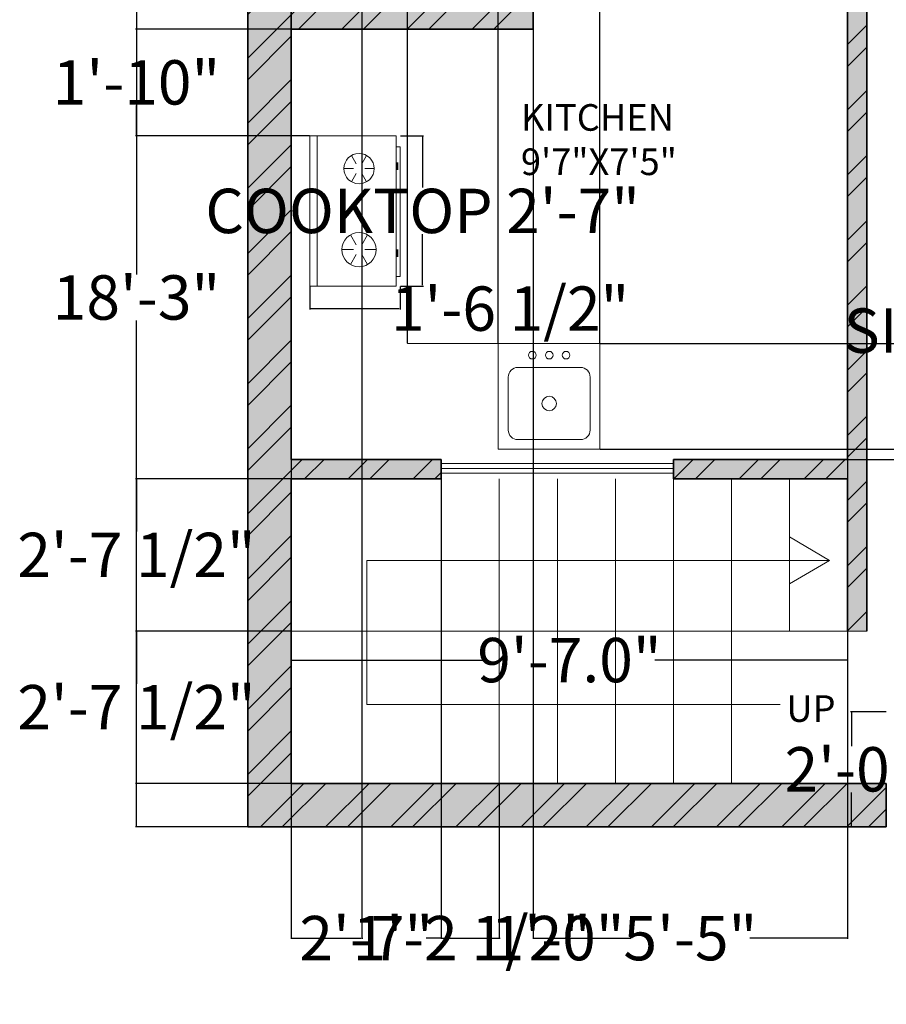
# Model space of a CAD drawing. Units: inches. Extents: x 1086 to 1540, y 3343 to 3848.
# Tile 1 of 8: x 1148 to 1327, y 3343 to 3547. Entities that reach past the tile are written whole.
import ezdxf

# ---------------------------------------------------------------- set-up
doc = ezdxf.new("R2010")
doc.units = ezdxf.units.IN
for name, color, linetype, lineweight in [('A-ANNO-DIMS', 2, 'Continuous', 13), ('A-ANNO-SYMB', 7, 'Continuous', 18), ('A-ANNO-TEXT', 7, 'Continuous', 18), ('A-AREA-IDEN', 7, 'Continuous', 18), ('A-EQPM', 8, 'Continuous', 18), ('A-FLOR-CASE', 8, 'Continuous', 18), ('A-FLOR-FIXT', 9, 'Continuous', 18), ('A-FLOR-STRS', 7, 'Continuous', 18), ('A-WALL-PATT', 252, 'Continuous', 9), ('A_TEXT_SMALL', 18, 'Continuous', 5), ('WALL', 7, 'Continuous', 35), ('WINDOW', 160, 'Continuous', 15)]:
    doc.layers.add(name, color=color, linetype=linetype, lineweight=lineweight)
doc.layers.add('FURN3D', color=229, linetype='Continuous', lineweight=5, true_color=0x4a3f41)
doc.styles.get("Standard").update_dxf_attribs({"font": 'arial.ttf'})
doc.dimstyles.get("Standard").update_dxf_attribs({"dimtxt": 9.18, "dimasz": 0.18, "dimexe": 0.18, "dimexo": 0.0625, "dimgap": 0.09, "dimtad": 0, "dimtih": 1, "dimtoh": 1, "dimdec": 1, "dimzin": 0, "dimdsep": 46, "dimlunit": 3, "dimtxsty": 'Standard', "dimcen": 0.09, "dimadec": 0, "dimazin": 0, "dimtfac": 1, "dimtdec": 1, "dimtofl": 0, "dimtmove": 0, "dimatfit": 3, "dimfxl": 1, "dimtolj": 1, "dimtzin": 0, "dimarcsym": 0})

# ---------------------------------------------------------------- blocks, each defined once
blk = doc.blocks.new('A$C21540130')
at = {"layer": 'FURN3D'}
for p, q in [((1.57, 0), (1.57, 31.11)), ((9.61, 25.31), (8.63, 27.01)), ((10.79, 25.31), (11.77, 27.01)), ((9.02, 24.29, -27.54), (7.06, 24.29, -27.54)), ((9.61, 23.27), (8.63, 21.57)), ((10.79, 23.27), (11.77, 21.57)), ((11.38, 24.29, -27.54), (13.34, 24.29, -27.54)), ((9.61, 8.56), (8.43, 10.6)), ((10.79, 8.56), (11.97, 10.6)), ((9.02, 7.54), (6.67, 7.54)), ((9.61, 6.52), (8.43, 4.48)), ((10.79, 6.52), (11.97, 4.48)), ((11.38, 7.54), (13.73, 7.54))]:
    blk.add_line(p, q, dxfattribs=at)
for points in [[(0, 0), (0, 31.11), (17.9, 31.11), (17.9, 0)], [(18.68, 1.96), (18.68, 28.83), (17.9, 28.83), (17.9, 1.96)]]:
    blk.add_lwpolyline(points, close=True, dxfattribs=at)
for centre, radius in [((10.2, 24.29), 3.14), ((10.2, 7.54), 3.53)]:
    blk.add_circle(centre, radius, dxfattribs=at)
for points in [[(17.9, 24.03), (18.29, 24.03), (17.9, 25.6), (18.29, 25.6)], [(17.9, 6.05), (18.29, 6.05), (17.9, 7.62), (18.29, 7.62)]]:
    blk.add_solid(points, dxfattribs=at)
blk = doc.blocks.new('reh-flat-2')
at = {"layer": 'A_TEXT_SMALL'}
for p, q in [((486053827.2, -394630231.2), (486054182.4, -394629799.8)), ((486054182.4, -394629799.8), (486054596.6, -394630140.9)), ((486053979.5, -394630126.3), (486054157.1, -394629910.6)), ((486054228.6, -394629903.6), (486054483.5, -394630113.5)), ((486054596.6, -394630140.9), (486054241.4, -394630572.3)), ((486054241.3, -394630407.7), (486053986.4, -394630197.8)), ((486054490.4, -394630185), (486054312.8, -394630400.7)), ((486054241.4, -394630572.3), (486053827.2, -394630231.2))]:
    blk.add_line(p, q, dxfattribs=at)
for centre, radius in [((486054234.9, -394630155.7), 38.1), ((486054004.1, -394630296.2), 20.1), ((486054072.7, -394630352.7), 20.1), ((486054141.4, -394630409.3), 20.1)]:
    blk.add_circle(centre, radius, dxfattribs=at)
for centre, start, end in [((486054196.3, -394629942.9), 50.5305, 140.5305), ((486054451.2, -394630152.8), 320.5305, 50.5305), ((486054018.7, -394630158.5), 140.5305, 230.5305), ((486054273.6, -394630368.4), 230.5305, 320.5305)]:
    blk.add_arc(centre, 50.8, start, end, dxfattribs=at)
blk = doc.blocks.new('*D16')
at = {"layer": 'A-ANNO-DIMS', "color": 0, "lineweight": -2, "transparency": 16777216}
for p, q in [((1203.74, 3420.01), (1203.74, 3413.89)), ((1318.74, 3420.01), (1318.74, 3413.89)), ((1203.92, 3414.07), (1243.6, 3414.07)), ((1318.56, 3414.07), (1278.88, 3414.07))]:
    blk.add_line(p, q, dxfattribs=at)
at = {"layer": 'A-ANNO-DIMS', "color": 0, "transparency": 16777216}
for points in [[(1203.92, 3414.1), (1203.92, 3414.04), (1203.74, 3414.07)], [(1318.56, 3414.1), (1318.56, 3414.04), (1318.74, 3414.07)]]:
    blk.add_solid(points, dxfattribs=at)
at = {"layer": 'Defpoints', "color": 0, "transparency": 16777216}
for p in [(1203.74, 3420.07), (1318.74, 3420.07), (1318.74, 3414.07)]:
    blk.add_point(p, dxfattribs=at)
at = {"layer": 'A-ANNO-DIMS', "color": 0, "transparency": 16777216, "insert": (1261.24, 3414.07), "char_height": 9.18, "attachment_point": 5}
blk.add_mtext('\\A1;9\'-7.0"', dxfattribs=at)
blk = doc.blocks.new('WIN-GLAZING-48IN')
for p, q in [((48, 1), (0, 1)), ((48, 0), (0, 0)), ((48, -1), (0, -1))]:
    blk.add_line(p, q)
blk = doc.blocks.new('*D29')
at = {"layer": 'A-ANNO-DIMS', "color": 0, "lineweight": -2, "transparency": 16777216}
for p, q in [((1387.77, 3493.16), (1384.37, 3493.16)), ((1384.55, 3492.98), (1384.55, 3487.04)), ((1384.55, 3471.44), (1384.55, 3477.37)), ((1387.77, 3471.26), (1384.37, 3471.26))]:
    blk.add_line(p, q, dxfattribs=at)
at = {"layer": 'A-ANNO-DIMS', "color": 0, "transparency": 16777216}
for points in [[(1384.52, 3492.98), (1384.58, 3492.98), (1384.55, 3493.16)], [(1384.52, 3471.44), (1384.58, 3471.44), (1384.55, 3471.26)]]:
    blk.add_solid(points, dxfattribs=at)
at = {"layer": 'Defpoints', "color": 0, "transparency": 16777216}
for p in [(1384.55, 3493.16), (1387.83, 3493.16), (1387.83, 3471.26)]:
    blk.add_point(p, dxfattribs=at)
at = {"layer": 'A-ANNO-DIMS', "color": 0, "transparency": 16777216, "insert": (1384.55, 3482.21), "char_height": 9.18, "attachment_point": 5}
blk.add_mtext('\\A1;SIDE TABLE 1\'-10" TYP.', dxfattribs=at)
blk = doc.blocks.new('*D39')
at = {"layer": 'A-ANNO-DIMS', "color": 0, "lineweight": -2, "transparency": 16777216}
for p, q in [((1226.3, 3522.53), (1231.08, 3522.53)), ((1230.9, 3522.35), (1230.9, 3511.81)), ((1230.9, 3491.6), (1230.9, 3502.13)), ((1226.3, 3491.42), (1231.08, 3491.42))]:
    blk.add_line(p, q, dxfattribs=at)
at = {"layer": 'A-ANNO-DIMS', "color": 0, "transparency": 16777216}
for points in [[(1230.87, 3522.35), (1230.93, 3522.35), (1230.9, 3522.53)], [(1230.87, 3491.6), (1230.93, 3491.6), (1230.9, 3491.42)]]:
    blk.add_solid(points, dxfattribs=at)
at = {"layer": 'Defpoints', "color": 0, "transparency": 16777216}
for p in [(1226.24, 3522.53), (1230.9, 3522.53), (1226.24, 3491.42)]:
    blk.add_point(p, dxfattribs=at)
at = {"layer": 'A-ANNO-DIMS', "color": 0, "transparency": 16777216, "insert": (1230.9, 3506.97), "char_height": 9.18, "attachment_point": 5}
blk.add_mtext('\\A1;COOKTOP 2\'-7"', dxfattribs=at)
blk = doc.blocks.new('*D40')
at = {"layer": 'A-ANNO-DIMS', "color": 0, "lineweight": -2, "transparency": 16777216}
for p, q in [((1207.55, 3491.36), (1207.55, 3486.58)), ((1226.24, 3491.36), (1226.24, 3486.58)), ((1207.73, 3486.76), (1226.06, 3486.76)), ((1226.24, 3486.76), (1226.42, 3486.76))]:
    blk.add_line(p, q, dxfattribs=at)
at = {"layer": 'A-ANNO-DIMS', "color": 0, "transparency": 16777216}
for points in [[(1207.73, 3486.79), (1207.73, 3486.73), (1207.55, 3486.76)], [(1226.06, 3486.79), (1226.06, 3486.73), (1226.24, 3486.76)]]:
    blk.add_solid(points, dxfattribs=at)
at = {"layer": 'Defpoints', "color": 0, "transparency": 16777216}
for p in [(1207.55, 3491.42), (1226.24, 3491.42), (1226.24, 3486.76)]:
    blk.add_point(p, dxfattribs=at)
at = {"layer": 'A-ANNO-DIMS', "color": 0, "transparency": 16777216, "insert": (1248.97, 3486.76), "char_height": 9.18, "attachment_point": 5}
blk.add_mtext('\\A1;1\'-6 1/2"', dxfattribs=at)
blk = doc.blocks.new('*D44')
at = {"layer": 'A-ANNO-DIMS', "color": 0, "lineweight": -2, "transparency": 16777216}
for p, q in [((1326.68, 3403.39), (1319.36, 3403.39)), ((1319.54, 3403.21), (1319.54, 3396.26)), ((1319.54, 3379.75), (1319.54, 3386.7)), ((1326.68, 3379.57), (1319.36, 3379.57))]:
    blk.add_line(p, q, dxfattribs=at)
at = {"layer": 'A-ANNO-DIMS', "color": 0, "transparency": 16777216}
for points in [[(1319.51, 3403.21), (1319.57, 3403.21), (1319.54, 3403.39)], [(1319.51, 3379.75), (1319.57, 3379.75), (1319.54, 3379.57)]]:
    blk.add_solid(points, dxfattribs=at)
at = {"layer": 'Defpoints', "color": 0, "transparency": 16777216}
for p in [(1326.74, 3403.39), (1319.54, 3379.57), (1326.74, 3379.57)]:
    blk.add_point(p, dxfattribs=at)
at = {"layer": 'A-ANNO-DIMS', "color": 0, "transparency": 16777216, "insert": (1319.54, 3391.48), "char_height": 9.18, "attachment_point": 5}
blk.add_mtext('\\A1;2\'-0"', dxfattribs=at)
blk = doc.blocks.new('*D52')
at = {"layer": 'A-ANNO-DIMS', "color": 0, "lineweight": -2, "transparency": 16777216}
for p, q in [((1194.68, 3598.57), (1171.56, 3598.57)), ((1171.74, 3598.39), (1171.74, 3493.85)), ((1171.74, 3379.75), (1171.74, 3484.29)), ((1194.68, 3379.57), (1171.56, 3379.57))]:
    blk.add_line(p, q, dxfattribs=at)
at = {"layer": 'A-ANNO-DIMS', "color": 0, "transparency": 16777216}
for points in [[(1171.71, 3598.39), (1171.77, 3598.39), (1171.74, 3598.57)], [(1171.71, 3379.75), (1171.77, 3379.75), (1171.74, 3379.57)]]:
    blk.add_solid(points, dxfattribs=at)
at = {"layer": 'Defpoints', "color": 0, "transparency": 16777216}
for p in [(1171.74, 3598.57), (1194.74, 3598.57), (1194.74, 3379.57)]:
    blk.add_point(p, dxfattribs=at)
at = {"layer": 'A-ANNO-DIMS', "color": 0, "transparency": 16777216, "insert": (1171.74, 3489.07), "char_height": 9.18, "attachment_point": 5}
blk.add_mtext('\\A1;18\'-3"', dxfattribs=at)
blk = doc.blocks.new('*D54')
at = {"layer": 'A-ANNO-DIMS', "color": 0, "lineweight": -2, "transparency": 16777216}
for p, q in [((1203.74, 3451.51), (1203.74, 3356.39)), ((1234.74, 3451.51), (1234.74, 3356.39)), ((1203.92, 3356.57), (1206.87, 3356.57)), ((1234.56, 3356.57), (1231.61, 3356.57))]:
    blk.add_line(p, q, dxfattribs=at)
at = {"layer": 'A-ANNO-DIMS', "color": 0, "transparency": 16777216}
for points in [[(1203.92, 3356.6), (1203.92, 3356.54), (1203.74, 3356.57)], [(1234.56, 3356.6), (1234.56, 3356.54), (1234.74, 3356.57)]]:
    blk.add_solid(points, dxfattribs=at)
at = {"layer": 'Defpoints', "color": 0, "transparency": 16777216}
for p in [(1203.74, 3451.57), (1234.74, 3451.57), (1234.74, 3356.57)]:
    blk.add_point(p, dxfattribs=at)
at = {"layer": 'A-ANNO-DIMS', "color": 0, "transparency": 16777216, "insert": (1219.24, 3356.57), "char_height": 9.18, "attachment_point": 5}
blk.add_mtext('\\A1;2\'-7"', dxfattribs=at)
blk = doc.blocks.new('*D55')
at = {"layer": 'A-ANNO-DIMS', "color": 0, "lineweight": -2, "transparency": 16777216}
for p, q in [((1203.74, 3634.51), (1203.74, 3356.39)), ((1218.33, 3634.51), (1218.33, 3356.39)), ((1203.92, 3356.57), (1218.15, 3356.57)), ((1218.33, 3356.57), (1218.51, 3356.57))]:
    blk.add_line(p, q, dxfattribs=at)
at = {"layer": 'A-ANNO-DIMS', "color": 0, "transparency": 16777216}
for points in [[(1203.92, 3356.6), (1203.92, 3356.54), (1203.74, 3356.57)], [(1218.15, 3356.6), (1218.15, 3356.54), (1218.33, 3356.57)]]:
    blk.add_solid(points, dxfattribs=at)
at = {"layer": 'Defpoints', "color": 0, "transparency": 16777216}
for p in [(1203.74, 3634.57), (1218.33, 3634.57), (1218.33, 3356.57)]:
    blk.add_point(p, dxfattribs=at)
at = {"layer": 'A-ANNO-DIMS', "color": 0, "transparency": 16777216, "insert": (1241.07, 3356.57), "char_height": 9.18, "attachment_point": 5}
blk.add_mtext('\\A1;1\'-2 1/2"', dxfattribs=at)
blk = doc.blocks.new('*D56')
at = {"layer": 'A-ANNO-DIMS', "color": 0, "lineweight": -2, "transparency": 16777216}
for p, q in [((1203.74, 3544.63), (1203.74, 3834.75)), ((1203.92, 3834.57), (1227.56, 3834.57)), ((1227.74, 3544.63), (1227.74, 3834.75)), ((1227.74, 3834.57), (1227.92, 3834.57))]:
    blk.add_line(p, q, dxfattribs=at)
at = {"layer": 'A-ANNO-DIMS', "color": 0, "transparency": 16777216}
for points in [[(1203.92, 3834.6), (1203.92, 3834.54), (1203.74, 3834.57)], [(1227.56, 3834.6), (1227.56, 3834.54), (1227.74, 3834.57)]]:
    blk.add_solid(points, dxfattribs=at)
at = {"layer": 'Defpoints', "color": 0, "transparency": 16777216}
for p in [(1227.74, 3834.57), (1203.74, 3544.57), (1227.74, 3544.57)]:
    blk.add_point(p, dxfattribs=at)
at = {"layer": 'A-ANNO-DIMS', "color": 0, "transparency": 16777216, "insert": (1240.29, 3834.57), "char_height": 9.18, "attachment_point": 5}
blk.add_mtext('\\A1;2\'-0"', dxfattribs=at)
blk = doc.blocks.new('*D57')
at = {"layer": 'A-ANNO-DIMS', "color": 0, "lineweight": -2, "transparency": 16777216}
for p, q in [((1318.8, 3479.57), (1493.92, 3479.57)), ((1493.74, 3479.39), (1493.74, 3472.35)), ((1493.74, 3455.75), (1493.74, 3462.79)), ((1318.8, 3455.57), (1493.92, 3455.57))]:
    blk.add_line(p, q, dxfattribs=at)
at = {"layer": 'A-ANNO-DIMS', "color": 0, "transparency": 16777216}
for points in [[(1493.71, 3479.39), (1493.77, 3479.39), (1493.74, 3479.57)], [(1493.71, 3455.75), (1493.77, 3455.75), (1493.74, 3455.57)]]:
    blk.add_solid(points, dxfattribs=at)
at = {"layer": 'Defpoints', "color": 0, "transparency": 16777216}
for p in [(1318.74, 3479.57), (1493.74, 3479.57), (1318.74, 3455.57)]:
    blk.add_point(p, dxfattribs=at)
at = {"layer": 'A-ANNO-DIMS', "color": 0, "transparency": 16777216, "insert": (1493.74, 3467.57), "char_height": 9.18, "attachment_point": 5}
blk.add_mtext('\\A1;2\'-0"', dxfattribs=at)
blk = doc.blocks.new('*D58')
at = {"layer": 'A-ANNO-DIMS', "color": 0, "lineweight": -2, "transparency": 16777216}
for p, q in [((1246.48, 3479.63), (1246.48, 3834.75)), ((1246.66, 3834.57), (1267.34, 3834.57)), ((1267.52, 3479.63), (1267.52, 3834.75)), ((1267.52, 3834.57), (1267.7, 3834.57))]:
    blk.add_line(p, q, dxfattribs=at)
at = {"layer": 'A-ANNO-DIMS', "color": 0, "transparency": 16777216}
for points in [[(1246.66, 3834.6), (1246.66, 3834.54), (1246.48, 3834.57)], [(1267.34, 3834.6), (1267.34, 3834.54), (1267.52, 3834.57)]]:
    blk.add_solid(points, dxfattribs=at)
at = {"layer": 'Defpoints', "color": 0, "transparency": 16777216}
for p in [(1267.52, 3834.57), (1246.48, 3479.57), (1267.52, 3479.57)]:
    blk.add_point(p, dxfattribs=at)
at = {"layer": 'A-ANNO-DIMS', "color": 0, "transparency": 16777216, "insert": (1279.55, 3834.57), "char_height": 9.18, "attachment_point": 5}
blk.add_mtext('\\A1;1\'-9"', dxfattribs=at)
blk = doc.blocks.new('*D59')
at = {"layer": 'A-ANNO-DIMS', "color": 0, "lineweight": -2, "transparency": 16777216}
for p, q in [((1267.58, 3479.57), (1493.92, 3479.57)), ((1493.74, 3479.39), (1493.74, 3473.4)), ((1493.74, 3457.85), (1493.74, 3463.84)), ((1267.58, 3457.67), (1493.92, 3457.67))]:
    blk.add_line(p, q, dxfattribs=at)
at = {"layer": 'A-ANNO-DIMS', "color": 0, "transparency": 16777216}
for points in [[(1493.71, 3479.39), (1493.77, 3479.39), (1493.74, 3479.57)], [(1493.71, 3457.85), (1493.77, 3457.85), (1493.74, 3457.67)]]:
    blk.add_solid(points, dxfattribs=at)
at = {"layer": 'Defpoints', "color": 0, "transparency": 16777216}
for p in [(1267.52, 3479.57), (1493.74, 3479.57), (1267.52, 3457.67)]:
    blk.add_point(p, dxfattribs=at)
at = {"layer": 'A-ANNO-DIMS', "color": 0, "transparency": 16777216, "insert": (1493.74, 3468.62), "char_height": 9.18, "attachment_point": 5}
blk.add_mtext('\\A1;1\'-10"', dxfattribs=at)
blk = doc.blocks.new('*D60')
at = {"layer": 'A-ANNO-DIMS', "color": 0, "lineweight": -2, "transparency": 16777216}
for p, q in [((1227.74, 3479.63), (1227.74, 3834.75)), ((1227.92, 3834.57), (1246.3, 3834.57)), ((1246.48, 3479.63), (1246.48, 3834.75)), ((1246.48, 3834.57), (1246.66, 3834.57))]:
    blk.add_line(p, q, dxfattribs=at)
at = {"layer": 'A-ANNO-DIMS', "color": 0, "transparency": 16777216}
for points in [[(1227.92, 3834.6), (1227.92, 3834.54), (1227.74, 3834.57)], [(1246.3, 3834.6), (1246.3, 3834.54), (1246.48, 3834.57)]]:
    blk.add_solid(points, dxfattribs=at)
at = {"layer": 'Defpoints', "color": 0, "transparency": 16777216}
for p in [(1246.48, 3834.57), (1227.74, 3479.57), (1246.48, 3479.57)]:
    blk.add_point(p, dxfattribs=at)
at = {"layer": 'A-ANNO-DIMS', "color": 0, "transparency": 16777216, "insert": (1269.22, 3834.57), "char_height": 9.18, "attachment_point": 5}
blk.add_mtext('\\A1;1\'-6 1/2"', dxfattribs=at)
blk = doc.blocks.new('*D61')
at = {"layer": 'A-ANNO-DIMS', "color": 0, "lineweight": -2, "transparency": 16777216}
for p, q in [((1203.68, 3544.57), (1171.56, 3544.57)), ((1171.74, 3544.39), (1171.74, 3538.33)), ((1171.74, 3522.71), (1171.74, 3528.77)), ((1207.49, 3522.53), (1171.56, 3522.53))]:
    blk.add_line(p, q, dxfattribs=at)
at = {"layer": 'A-ANNO-DIMS', "color": 0, "transparency": 16777216}
for points in [[(1171.71, 3544.39), (1171.77, 3544.39), (1171.74, 3544.57)], [(1171.71, 3522.71), (1171.77, 3522.71), (1171.74, 3522.53)]]:
    blk.add_solid(points, dxfattribs=at)
at = {"layer": 'Defpoints', "color": 0, "transparency": 16777216}
for p in [(1171.74, 3544.57), (1203.74, 3544.57), (1207.55, 3522.53)]:
    blk.add_point(p, dxfattribs=at)
at = {"layer": 'A-ANNO-DIMS', "color": 0, "transparency": 16777216, "insert": (1171.74, 3533.55), "char_height": 9.18, "attachment_point": 5}
blk.add_mtext('\\A1;1\'-10"', dxfattribs=at)
blk = doc.blocks.new('*D62')
at = {"layer": 'A-ANNO-DIMS', "color": 0, "lineweight": -2, "transparency": 16777216}
for p, q in [((1203.68, 3420.07), (1171.56, 3420.07)), ((1171.74, 3419.89), (1171.74, 3409.16)), ((1171.74, 3388.75), (1171.74, 3399.48)), ((1203.68, 3388.57), (1171.56, 3388.57))]:
    blk.add_line(p, q, dxfattribs=at)
at = {"layer": 'A-ANNO-DIMS', "color": 0, "transparency": 16777216}
for points in [[(1171.71, 3419.89), (1171.77, 3419.89), (1171.74, 3420.07)], [(1171.71, 3388.75), (1171.77, 3388.75), (1171.74, 3388.57)]]:
    blk.add_solid(points, dxfattribs=at)
at = {"layer": 'Defpoints', "color": 0, "transparency": 16777216}
for p in [(1171.74, 3420.07), (1203.74, 3420.07), (1203.74, 3388.57)]:
    blk.add_point(p, dxfattribs=at)
at = {"layer": 'A-ANNO-DIMS', "color": 0, "transparency": 16777216, "insert": (1171.74, 3404.32), "char_height": 9.18, "attachment_point": 5}
blk.add_mtext('\\A1;2\'-7 1/2"', dxfattribs=at)
blk = doc.blocks.new('*D63')
at = {"layer": 'A-ANNO-DIMS', "color": 0, "lineweight": -2, "transparency": 16777216}
for p, q in [((1203.68, 3451.57), (1171.56, 3451.57)), ((1171.74, 3451.39), (1171.74, 3440.66)), ((1171.74, 3420.25), (1171.74, 3430.98)), ((1203.68, 3420.07), (1171.56, 3420.07))]:
    blk.add_line(p, q, dxfattribs=at)
at = {"layer": 'A-ANNO-DIMS', "color": 0, "transparency": 16777216}
for points in [[(1171.71, 3451.39), (1171.77, 3451.39), (1171.74, 3451.57)], [(1171.71, 3420.25), (1171.77, 3420.25), (1171.74, 3420.07)]]:
    blk.add_solid(points, dxfattribs=at)
at = {"layer": 'Defpoints', "color": 0, "transparency": 16777216}
for p in [(1171.74, 3451.57), (1203.74, 3451.57), (1203.74, 3420.07)]:
    blk.add_point(p, dxfattribs=at)
at = {"layer": 'A-ANNO-DIMS', "color": 0, "transparency": 16777216, "insert": (1171.74, 3435.82), "char_height": 9.18, "attachment_point": 5}
blk.add_mtext('\\A1;2\'-7 1/2"', dxfattribs=at)
blk = doc.blocks.new('*D64')
at = {"layer": 'A-ANNO-DIMS', "color": 0, "lineweight": -2, "transparency": 16777216}
for p, q in [((1234.74, 3388.51), (1234.74, 3356.39)), ((1246.74, 3388.51), (1246.74, 3356.39)), ((1234.92, 3356.57), (1246.56, 3356.57)), ((1246.74, 3356.57), (1246.92, 3356.57))]:
    blk.add_line(p, q, dxfattribs=at)
at = {"layer": 'A-ANNO-DIMS', "color": 0, "transparency": 16777216}
for points in [[(1234.92, 3356.6), (1234.92, 3356.54), (1234.74, 3356.57)], [(1246.56, 3356.6), (1246.56, 3356.54), (1246.74, 3356.57)]]:
    blk.add_solid(points, dxfattribs=at)
at = {"layer": 'Defpoints', "color": 0, "transparency": 16777216}
for p in [(1234.74, 3388.57), (1246.74, 3388.57), (1246.74, 3356.57)]:
    blk.add_point(p, dxfattribs=at)
at = {"layer": 'A-ANNO-DIMS', "color": 0, "transparency": 16777216, "insert": (1258.78, 3356.57), "char_height": 9.18, "attachment_point": 5}
blk.add_mtext('\\A1;1\'-0"', dxfattribs=at)
blk = doc.blocks.new('*D65')
at = {"layer": 'A-ANNO-DIMS', "color": 0, "lineweight": -2, "transparency": 16777216}
for p, q in [((1203.74, 3388.51), (1203.74, 3356.39)), ((1234.74, 3388.51), (1234.74, 3356.39)), ((1203.92, 3356.57), (1206.87, 3356.57)), ((1234.56, 3356.57), (1231.61, 3356.57))]:
    blk.add_line(p, q, dxfattribs=at)
at = {"layer": 'A-ANNO-DIMS', "color": 0, "transparency": 16777216}
for points in [[(1203.92, 3356.6), (1203.92, 3356.54), (1203.74, 3356.57)], [(1234.56, 3356.6), (1234.56, 3356.54), (1234.74, 3356.57)]]:
    blk.add_solid(points, dxfattribs=at)
at = {"layer": 'Defpoints', "color": 0, "transparency": 16777216}
for p in [(1203.74, 3388.57), (1234.74, 3388.57), (1234.74, 3356.57)]:
    blk.add_point(p, dxfattribs=at)
at = {"layer": 'A-ANNO-DIMS', "color": 0, "transparency": 16777216, "insert": (1219.24, 3356.57), "char_height": 9.18, "attachment_point": 5}
blk.add_mtext('\\A1;2\'-7"', dxfattribs=at)
blk = doc.blocks.new('*D72')
at = {"layer": 'A-ANNO-DIMS', "color": 0, "lineweight": -2, "transparency": 16777216}
for p, q in [((1318.74, 3548.51), (1318.74, 3356.39)), ((1253.74, 3544.51), (1253.74, 3356.39)), ((1253.92, 3356.57), (1273.95, 3356.57)), ((1318.56, 3356.57), (1298.53, 3356.57))]:
    blk.add_line(p, q, dxfattribs=at)
at = {"layer": 'A-ANNO-DIMS', "color": 0, "transparency": 16777216}
for points in [[(1253.92, 3356.6), (1253.92, 3356.54), (1253.74, 3356.57)], [(1318.56, 3356.6), (1318.56, 3356.54), (1318.74, 3356.57)]]:
    blk.add_solid(points, dxfattribs=at)
at = {"layer": 'Defpoints', "color": 0, "transparency": 16777216}
for p in [(1318.74, 3548.57), (1253.74, 3544.57), (1318.74, 3356.57)]:
    blk.add_point(p, dxfattribs=at)
at = {"layer": 'A-ANNO-DIMS', "color": 0, "transparency": 16777216, "insert": (1286.24, 3356.57), "char_height": 9.18, "attachment_point": 5}
blk.add_mtext('\\A1;5\'-5"', dxfattribs=at)

msp = doc.modelspace()

# ---------------------------------------------------------------- hatches: boundary and pattern name
at = {"layer": 'A-WALL-PATT'}
h = msp.add_hatch(dxfattribs=at)
h.set_pattern_fill('ANSI32', color=256)
h.paths.add_polyline_path([(1234.55, 3811.57), (1234.55, 3811.57), (1194.74, 3811.57), (1194.74, 3622.57), (1203.74, 3622.57), (1203.74, 3634.57), (1218.33, 3634.57), (1218.33, 3638.57), (1203.74, 3638.57), (1203.74, 3802.57), (1234.55, 3802.57)])
h.paths.add_polyline_path([(1371.06, 3811.57), (1371.06, 3811.57), (1282.55, 3811.57), (1282.55, 3802.57), (1331.74, 3802.57), (1331.74, 3634.57), (1335.74, 3634.57), (1335.74, 3639.57), (1335.74, 3802.57), (1371.06, 3802.57)])
h.paths.add_polyline_path([(1470.74, 3811.57), (1419.06, 3811.57), (1419.06, 3802.57), (1461.74, 3802.57), (1461.74, 3638.57), (1461.74, 3548.57), (1425.74, 3548.57), (1425.74, 3582.21), (1421.74, 3582.21), (1421.74, 3548.57), (1376.74, 3548.57), (1376.74, 3602.57), (1373.71, 3602.57), (1372.74, 3602.57), (1372.74, 3544.57), (1461.74, 3544.57), (1461.74, 3379.57), (1470.74, 3379.57)])
h.paths.add_polyline_path([(1203.74, 3582.57), (1295.74, 3582.57), (1295.74, 3586.57), (1203.74, 3586.57), (1203.74, 3598.57), (1194.74, 3598.57), (1194.74, 3379.57), (1326.74, 3379.57), (1326.74, 3388.57), (1322.74, 3388.57), (1203.74, 3388.57), (1203.74, 3451.57), (1234.74, 3451.57), (1234.74, 3455.57), (1203.74, 3455.57), (1203.74, 3479.57), (1203.74, 3544.57), (1227.74, 3544.57), (1253.74, 3544.57), (1253.74, 3548.57), (1203.74, 3548.57)])
h.paths.add_polyline_path([(1461.74, 3638.57), (1371.74, 3638.57), (1371.74, 3634.57), (1372.74, 3634.57), (1372.74, 3632.57), (1376.74, 3632.57), (1376.74, 3634.57), (1421.74, 3634.57), (1421.74, 3606.21), (1425.74, 3606.21), (1425.74, 3634.57), (1461.74, 3634.57)])
h.paths.add_polyline_path([(1295.74, 3638.57), (1266.33, 3638.57), (1266.33, 3634.57), (1292.74, 3634.57), (1295.74, 3634.57)])
h.paths.add_polyline_path([(1322.74, 3548.57), (1318.74, 3548.57), (1318.74, 3455.57), (1282.74, 3455.57), (1282.74, 3451.57), (1318.74, 3451.57), (1318.74, 3420.07), (1322.74, 3420.07)], flags=17)
at = {"layer": 'A-WALL-PATT', "transparency": 33554559}
h = msp.add_hatch(color=256, dxfattribs=at)
h.dxf.hatch_style = 1
h.paths.add_polyline_path([(1234.55, 3811.57), (1234.55, 3811.57), (1194.74, 3811.57), (1194.74, 3622.57), (1203.74, 3622.57), (1203.74, 3634.57), (1218.33, 3634.57), (1218.33, 3638.57), (1203.74, 3638.57), (1203.74, 3802.57), (1234.55, 3802.57)])
h.paths.add_polyline_path([(1371.06, 3811.57), (1371.06, 3811.57), (1282.55, 3811.57), (1282.55, 3802.57), (1331.74, 3802.57), (1331.74, 3634.57), (1335.74, 3634.57), (1335.74, 3639.57), (1335.74, 3802.57), (1371.06, 3802.57)])
h.paths.add_polyline_path([(1470.74, 3811.57), (1419.06, 3811.57), (1419.06, 3802.57), (1461.74, 3802.57), (1461.74, 3638.57), (1461.74, 3548.57), (1425.74, 3548.57), (1425.74, 3582.21), (1421.74, 3582.21), (1421.74, 3548.57), (1376.74, 3548.57), (1376.74, 3602.57), (1372.74, 3602.57), (1372.74, 3544.57), (1461.74, 3544.57), (1461.74, 3379.57), (1470.74, 3379.57)])
h.paths.add_polyline_path([(1203.74, 3544.57), (1227.74, 3544.57), (1253.74, 3544.57), (1253.74, 3548.57), (1203.74, 3548.57), (1203.74, 3582.57), (1295.74, 3582.57), (1295.74, 3586.57), (1203.74, 3586.57), (1203.74, 3598.57), (1194.74, 3598.57), (1194.74, 3379.57), (1326.74, 3379.57), (1326.74, 3388.57), (1322.74, 3388.57), (1203.74, 3388.57), (1203.74, 3451.57), (1234.74, 3451.57), (1234.74, 3455.57), (1203.74, 3455.57)])
h.paths.add_polyline_path([(1413.74, 3388.57), (1413.74, 3388.57), (1374.74, 3388.57), (1374.74, 3383.18), (1374.74, 3383.18), (1374.74, 3379.57), (1413.74, 3379.57)], flags=17)
h.paths.add_polyline_path([(1322.74, 3548.57), (1318.74, 3548.57), (1318.74, 3455.57), (1282.74, 3455.57), (1282.74, 3451.57), (1318.74, 3451.57), (1318.74, 3420.07), (1322.74, 3420.07)], flags=17)
h.paths.add_polyline_path([(1295.74, 3638.57), (1266.33, 3638.57), (1266.33, 3634.57), (1292.74, 3634.57), (1295.74, 3634.57)])
h.paths.add_polyline_path([(1461.74, 3638.57), (1371.74, 3638.57), (1371.74, 3634.57), (1372.74, 3634.57), (1372.74, 3632.57), (1376.74, 3632.57), (1376.74, 3634.57), (1421.74, 3634.57), (1421.74, 3606.21), (1425.74, 3606.21), (1425.74, 3634.57), (1461.74, 3634.57)])

# ---------------------------------------------------------------- linework, layer by layer
at = {"layer": 'A-ANNO-SYMB'}
for p, q in [((1315.03, 3434.7), (1306.74, 3439.59)), ((1306.74, 3439.59), (1315.03, 3434.7)), ((1219.36, 3404.89), (1219.36, 3434.7)), ((1219.36, 3434.7), (1315.03, 3434.7)), ((1315.03, 3434.7), (1306.74, 3429.82)), ((1306.74, 3429.82), (1315.03, 3434.7)), ((1304.82, 3404.89), (1219.36, 3404.89))]:
    msp.add_line(p, q, dxfattribs=at)
at = {"layer": 'A-FLOR-CASE'}
for p, q in [((1203.74, 3544.57), (1227.74, 3544.57)), ((1227.74, 3544.57), (1227.74, 3479.57)), ((1203.74, 3455.57), (1203.74, 3479.57)), ((1227.74, 3479.57), (1318.74, 3479.57))]:
    msp.add_line(p, q, dxfattribs=at)
at = {"layer": 'A-FLOR-STRS'}
for p, q in [((1234.74, 3388.57), (1234.74, 3451.57)), ((1246.74, 3388.57), (1246.74, 3451.57)), ((1258.74, 3388.57), (1258.74, 3451.57)), ((1270.74, 3388.57), (1270.74, 3451.57)), ((1282.74, 3388.57), (1282.74, 3451.57)), ((1294.74, 3388.57), (1294.74, 3451.57)), ((1306.74, 3420.07), (1306.74, 3451.57)), ((1203.74, 3420.07), (1322.74, 3420.07))]:
    msp.add_line(p, q, dxfattribs=at)
at = {"layer": 'WALL'}
for p, q in [((1194.74, 3379.57), (1194.74, 3598.57)), ((1253.74, 3544.57), (1253.74, 3582.57)), ((1318.74, 3455.57), (1318.74, 3548.57)), ((1322.74, 3420.07), (1322.74, 3548.57)), ((1203.74, 3544.57), (1253.74, 3544.57)), ((1203.74, 3455.57), (1203.74, 3544.57)), ((1203.74, 3455.57), (1234.74, 3455.57)), ((1234.74, 3451.57), (1234.74, 3455.57)), ((1282.74, 3455.57), (1318.74, 3455.57)), ((1282.74, 3451.57), (1282.74, 3455.57)), ((1203.74, 3388.57), (1203.74, 3451.57)), ((1203.74, 3451.57), (1234.74, 3451.57)), ((1282.74, 3451.57), (1318.74, 3451.57)), ((1318.74, 3420.07), (1318.74, 3451.57)), ((1322.74, 3388.57), (1203.74, 3388.57)), ((1326.74, 3388.57), (1322.74, 3388.57)), ((1326.74, 3379.57), (1326.74, 3388.57)), ((1326.74, 3379.57), (1194.74, 3379.57))]:
    msp.add_line(p, q, dxfattribs=at)

# ---------------------------------------------------------------- block references
at = {"layer": 'A-EQPM'}
msp.add_blockref('A$C21540130', (1207.55, 3491.42), dxfattribs=at)
at = {"layer": 'A-FLOR-FIXT', "xscale": 0.0391972730482577, "yscale": 0.0391972730482577, "zscale": 0.0391972730482577, "rotation": 219.4694759622485}
msp.add_blockref('reh-flat-2', (24541471.79, 173138.35), dxfattribs=at)
at = {"layer": 'WINDOW'}
msp.add_blockref('WIN-GLAZING-48IN', (1234.74, 3453.72), dxfattribs=at)

# ---------------------------------------------------------------- texts
at = {"layer": 'A-ANNO-TEXT', "insert": (1306.08, 3406.8), "char_height": 8, "attachment_point": 1}
msp.add_mtext_dynamic_manual_height_columns('{\\H0.6875x;UP}', width=58.9878, gutter_width=0, heights=[37.04], dxfattribs=at)
at = {"layer": 'A-AREA-IDEN', "insert": (1251.21, 3529.05), "char_height": 8, "attachment_point": 1}
msp.add_mtext_dynamic_manual_height_columns('{\\H0.6875x;KITCHEN\\P9\'7"X7\'5"}  ', width=58.9878, gutter_width=0, heights=[37.04], dxfattribs=at)

# ---------------------------------------------------------------- dimensions: what is measured, and where the dimension line sits
at = {"layer": 'A-ANNO-DIMS'}
for base, p1, p2, override, picture, middle in [((1246.48, 3834.57), (1227.74, 3479.57), (1246.48, 3479.57), {"dimdec": 1, "dimlfac": 1, "dimrnd": 0, "dimzin": 1, "dimdsep": 46, "dimlunit": 4, "dimfrac": 2}, '*D60', (1269.22, 3834.57)), ((1227.74, 3834.57), (1203.74, 3544.57), (1227.74, 3544.57), {"dimdec": 1, "dimlfac": 1, "dimrnd": 0, "dimzin": 1, "dimdsep": 46, "dimlunit": 4, "dimfrac": 2}, '*D56', (1240.29, 3834.57)), ((1267.52, 3834.57), (1246.48, 3479.57), (1267.52, 3479.57), {"dimdec": 1, "dimlfac": 1, "dimrnd": 0, "dimzin": 1, "dimdsep": 46, "dimlunit": 4, "dimfrac": 2}, '*D58', (1279.55, 3834.57)), ((1218.33, 3356.57), (1203.74, 3634.57), (1218.33, 3634.57), {"dimdec": 1, "dimlfac": 1, "dimrnd": 0, "dimzin": 1, "dimdsep": 46, "dimlunit": 4, "dimfrac": 2}, '*D55', (1241.07, 3356.57)), ((1318.74, 3356.57), (1253.74, 3544.57), (1318.74, 3548.57), {"dimdec": 1, "dimlfac": 1, "dimrnd": 0, "dimzin": 1, "dimdsep": 46, "dimlunit": 4, "dimfrac": 2}, '*D72', (1286.24, 3356.57)), ((1226.24, 3486.76), (1207.55, 3491.42), (1226.24, 3491.42), {"dimdec": 1, "dimlfac": 1, "dimrnd": 0, "dimzin": 1, "dimdsep": 46, "dimlunit": 4, "dimfrac": 2}, '*D40', (1248.97, 3486.76)), ((1234.74, 3356.57), (1203.74, 3451.57), (1234.74, 3451.57), {"dimdec": 1, "dimlfac": 1, "dimrnd": 0, "dimzin": 1, "dimdsep": 46, "dimlunit": 4, "dimfrac": 2}, '*D54', (1219.24, 3356.57)), ((1318.74, 3414.07), (1203.74, 3420.07), (1318.74, 3420.07), {"dimclrd": 0, "dimclre": 0, "dimclrt": 0}, '*D16', (1261.24, 3414.07)), ((1234.74, 3356.57), (1203.74, 3388.57), (1234.74, 3388.57), {"dimdec": 1, "dimlfac": 1, "dimrnd": 0, "dimzin": 1, "dimdsep": 46, "dimlunit": 4, "dimfrac": 2}, '*D65', (1219.24, 3356.57)), ((1246.74, 3356.57), (1234.74, 3388.57), (1246.74, 3388.57), {"dimdec": 1, "dimlfac": 1, "dimrnd": 0, "dimzin": 1, "dimdsep": 46, "dimlunit": 4, "dimfrac": 2}, '*D64', (1258.78, 3356.57))]:
    dim = msp.add_linear_dim(base=base, p1=p1, p2=p2, dimstyle='Standard', override=override, dxfattribs=at)
    dim.commit()
    dim.dimension.update_dxf_attribs({"geometry": picture, "text_midpoint": middle})
for base, p1, p2, angle, picture, middle in [((1171.74, 3598.57), (1194.74, 3379.57), (1194.74, 3598.57), 90, '*D52', (1171.74, 3489.07)), ((1171.74, 3544.57), (1207.55, 3522.53), (1203.74, 3544.57), 90, '*D61', (1171.74, 3533.55)), ((1493.74, 3479.57), (1267.52, 3457.67), (1267.52, 3479.57), 90, '*D59', (1493.74, 3468.62)), ((1493.74, 3479.57), (1318.74, 3455.57), (1318.74, 3479.57), 90, '*D57', (1493.74, 3467.57)), ((1171.74, 3451.57), (1203.74, 3420.07), (1203.74, 3451.57), 90, '*D63', (1171.74, 3435.82)), ((1171.74, 3420.07), (1203.74, 3388.57), (1203.74, 3420.07), 90, '*D62', (1171.74, 3404.32)), ((1319.54, 3379.57), (1326.74, 3403.39), (1326.74, 3379.57), 270, '*D44', (1319.54, 3391.48))]:
    dim = msp.add_linear_dim(base=base, p1=p1, p2=p2, angle=angle, dimstyle='Standard', override={"dimdec": 1, "dimlfac": 1, "dimrnd": 0, "dimzin": 1, "dimdsep": 46, "dimlunit": 4, "dimfrac": 2}, dxfattribs=at)
    dim.commit()
    dim.dimension.update_dxf_attribs({"geometry": picture, "text_midpoint": middle})
for base, p1, p2, text, picture, middle in [((1230.9, 3522.53), (1226.24, 3491.42), (1226.24, 3522.53), 'COOKTOP <>', '*D39', (1230.9, 3506.97)), ((1384.55, 3493.16), (1387.83, 3471.26), (1387.83, 3493.16), 'SIDE TABLE <> TYP.', '*D29', (1384.55, 3482.21))]:
    dim = msp.add_linear_dim(base=base, p1=p1, p2=p2, angle=90, text=text, dimstyle='Standard', override={"dimdec": 1, "dimlfac": 1, "dimrnd": 0, "dimzin": 1, "dimdsep": 46, "dimlunit": 4, "dimfrac": 2}, dxfattribs=at)
    dim.commit()
    dim.dimension.update_dxf_attribs({"geometry": picture, "text_midpoint": middle})

doc.saveas('drawing.dxf')
